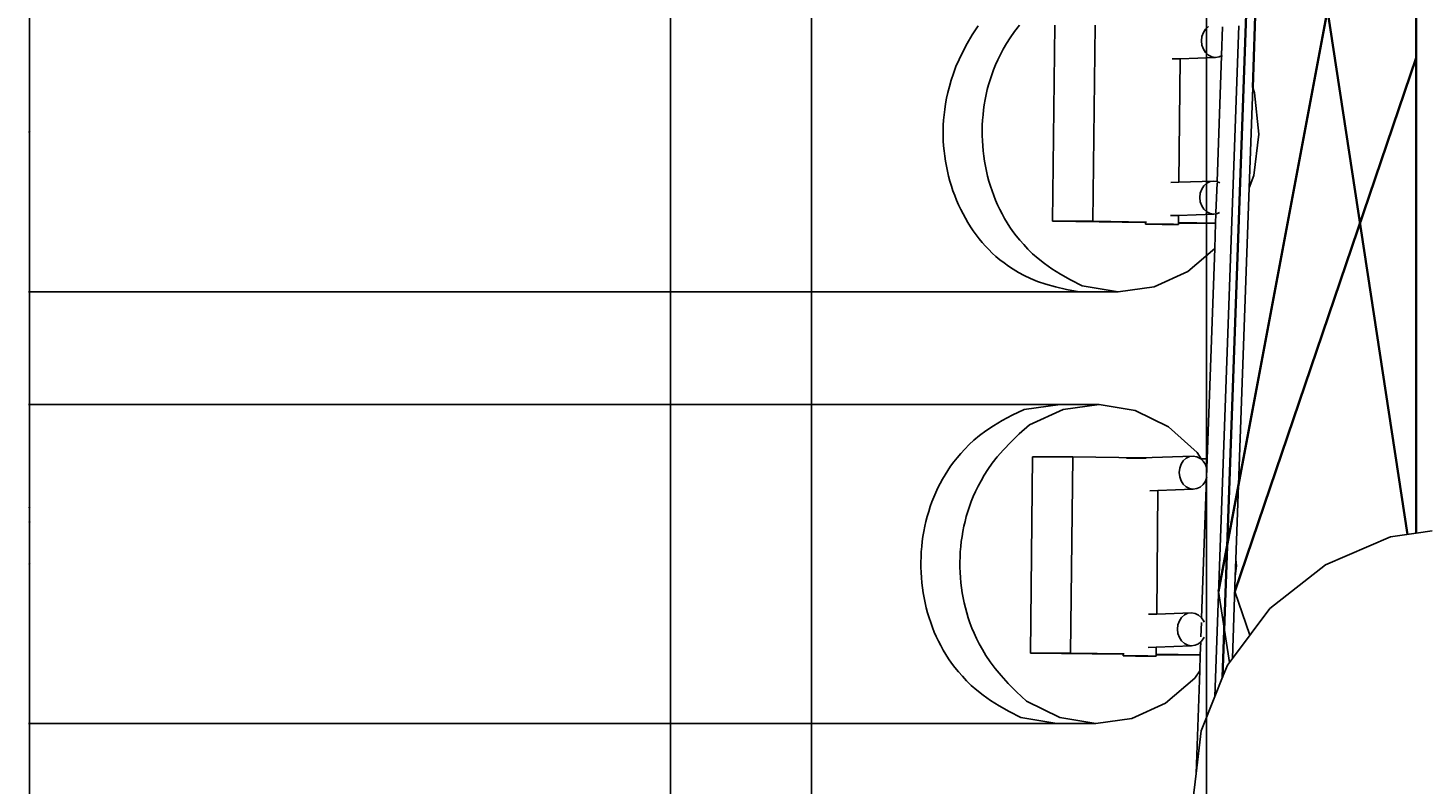
# Model space of a CAD drawing. Units: inches. Extents: x 3780 to 4301, y 1637 to 4224.
# Tile 5 of 8: x 3781 to 4040, y 3542 to 3682. Entities that reach past the tile are written whole.
import ezdxf

# ---------------------------------------------------------------- set-up
doc = ezdxf.new("R2010")
doc.units = ezdxf.units.IN
for name, color, linetype, lineweight in [('A-ANNO-DIMS', 2, 'Continuous', 18), ('E-COMM-DISH', 3, 'Continuous', 25), ('S-TOWR', 7, 'Continuous', 35)]:
    doc.layers.add(name, color=color, linetype=linetype, lineweight=lineweight)
doc.styles.get("Standard").update_dxf_attribs({"font": 'arial.ttf'})
doc.dimstyles.get("Standard").update_dxf_attribs({"dimtxt": 0.18, "dimasz": 0.18, "dimexe": 0.18, "dimexo": 0.0625, "dimgap": 0.09, "dimtad": 0, "dimtih": 1, "dimtoh": 1, "dimdec": 4, "dimzin": 0, "dimdsep": 46, "dimtxsty": 'Standard', "dimcen": 0.09, "dimadec": 0, "dimazin": 0, "dimtfac": 1, "dimtdec": 4, "dimtofl": 0, "dimtmove": 0, "dimatfit": 3, "dimfxl": 1, "dimtolj": 1, "dimtzin": 0, "dimarcsym": 0})

# ---------------------------------------------------------------- blocks, each defined once
blk = doc.blocks.new('*D11')
at = {"layer": 'A-ANNO-DIMS', "color": 0, "lineweight": -2, "transparency": 16777216}
for p, q in [((3916.19, 4105.28), (3780.66, 4105.28)), ((3780.84, 4105.1), (3780.84, 2930.44)), ((3780.84, 1755.43), (3780.84, 2930.08)), ((3934.09, 1755.25), (3780.66, 1755.25))]:
    blk.add_line(p, q, dxfattribs=at)
at = {"layer": 'A-ANNO-DIMS', "color": 0, "transparency": 16777216}
for points in [[(3780.81, 4105.1), (3780.87, 4105.1), (3780.84, 4105.28)], [(3780.81, 1755.43), (3780.87, 1755.43), (3780.84, 1755.25)]]:
    blk.add_solid(points, dxfattribs=at)
at = {"layer": 'Defpoints', "color": 0, "transparency": 16777216}
for p in [(3780.84, 4105.28), (3916.25, 4105.28), (3934.15, 1755.25)]:
    blk.add_point(p, dxfattribs=at)
at = {"layer": 'A-ANNO-DIMS', "color": 0, "transparency": 16777216, "insert": (3780.84, 2930.26), "char_height": 0.18, "attachment_point": 5}
blk.add_mtext('\\A1;2350', dxfattribs=at)
blk = doc.blocks.new('*D21')
at = {"layer": 'A-ANNO-DIMS', "color": 0, "lineweight": -2, "transparency": 16777216}
for p, q in [((4010.55, 3901.46), (4300.89, 3901.46)), ((4300.71, 3901.28), (4300.71, 3685.65)), ((4300.71, 3469.64), (4300.71, 3685.28)), ((4044.72, 3469.46), (4300.89, 3469.46))]:
    blk.add_line(p, q, dxfattribs=at)
at = {"layer": 'A-ANNO-DIMS', "color": 0, "transparency": 16777216}
for points in [[(4300.68, 3901.28), (4300.74, 3901.28), (4300.71, 3901.46)], [(4300.68, 3469.64), (4300.74, 3469.64), (4300.71, 3469.46)]]:
    blk.add_solid(points, dxfattribs=at)
at = {"layer": 'Defpoints', "color": 0, "transparency": 16777216}
for p in [(4010.49, 3901.46), (4300.71, 3901.46), (4044.66, 3469.46)]:
    blk.add_point(p, dxfattribs=at)
at = {"layer": 'A-ANNO-DIMS', "color": 0, "transparency": 16777216, "insert": (4300.71, 3685.46), "char_height": 0.18, "attachment_point": 5}
blk.add_mtext('\\A1;432', dxfattribs=at)
blk = doc.blocks.new('*D22')
at = {"layer": 'A-ANNO-DIMS', "color": 0, "lineweight": -2, "transparency": 16777216}
for p, q in [((3900.05, 3694.01), (3900.05, 1636.57)), ((4181.5, 3694.01), (4181.5, 1636.57)), ((3900.23, 1636.75), (4040.31, 1636.75)), ((4181.32, 1636.75), (4041.24, 1636.75))]:
    blk.add_line(p, q, dxfattribs=at)
at = {"layer": 'A-ANNO-DIMS', "color": 0, "transparency": 16777216}
for points in [[(3900.23, 1636.78), (3900.23, 1636.72), (3900.05, 1636.75)], [(4181.32, 1636.78), (4181.32, 1636.72), (4181.5, 1636.75)]]:
    blk.add_solid(points, dxfattribs=at)
at = {"layer": 'Defpoints', "color": 0, "transparency": 16777216}
for p in [(3900.05, 3694.07), (4181.5, 3694.07), (4181.5, 1636.75)]:
    blk.add_point(p, dxfattribs=at)
at = {"layer": 'A-ANNO-DIMS', "color": 0, "transparency": 16777216, "insert": (4040.77, 1636.75), "char_height": 0.18, "attachment_point": 5}
blk.add_mtext('\\A1;281.45', dxfattribs=at)
blk = doc.blocks.new('*D28')
at = {"layer": 'A-ANNO-DIMS', "color": 0, "lineweight": -2, "transparency": 16777216}
for p, q in [((3926.17, 3691.91), (3780.66, 3691.91)), ((3780.84, 3691.73), (3780.84, 3590.48)), ((3780.84, 3488.87), (3780.84, 3590.12)), ((4048.31, 3488.69), (3780.66, 3488.69))]:
    blk.add_line(p, q, dxfattribs=at)
at = {"layer": 'A-ANNO-DIMS', "color": 0, "transparency": 16777216}
for points in [[(3780.81, 3691.73), (3780.87, 3691.73), (3780.84, 3691.91)], [(3780.81, 3488.87), (3780.87, 3488.87), (3780.84, 3488.69)]]:
    blk.add_solid(points, dxfattribs=at)
at = {"layer": 'Defpoints', "color": 0, "transparency": 16777216}
for p in [(3780.84, 3691.91), (3926.23, 3691.91), (4048.37, 3488.69)]:
    blk.add_point(p, dxfattribs=at)
at = {"layer": 'A-ANNO-DIMS', "color": 0, "transparency": 16777216, "insert": (3780.84, 3590.3), "char_height": 0.18, "attachment_point": 5}
blk.add_mtext('\\A1;203.2', dxfattribs=at)
blk = doc.blocks.new('*D43')
at = {"layer": 'A-ANNO-DIMS', "color": 0, "lineweight": -2, "transparency": 16777216}
for p, q in [((3983.82, 3692.42), (3780.66, 3692.42)), ((3780.84, 3692.24), (3780.84, 3662.96)), ((3780.84, 3633.31), (3780.84, 3662.6)), ((3983.19, 3633.13), (3780.66, 3633.13))]:
    blk.add_line(p, q, dxfattribs=at)
at = {"layer": 'A-ANNO-DIMS', "color": 0, "transparency": 16777216}
for points in [[(3780.81, 3692.24), (3780.87, 3692.24), (3780.84, 3692.42)], [(3780.81, 3633.31), (3780.87, 3633.31), (3780.84, 3633.13)]]:
    blk.add_solid(points, dxfattribs=at)
at = {"layer": 'Defpoints', "color": 0, "transparency": 16777216}
for p in [(3983.89, 3692.42), (3780.84, 3633.13), (3983.25, 3633.13)]:
    blk.add_point(p, dxfattribs=at)
at = {"layer": 'A-ANNO-DIMS', "color": 0, "transparency": 16777216, "insert": (3780.84, 3662.78), "char_height": 0.18, "attachment_point": 5}
blk.add_mtext('\\A1;59.29', dxfattribs=at)
blk = doc.blocks.new('*D44')
at = {"layer": 'A-ANNO-DIMS', "color": 0, "lineweight": -2, "transparency": 16777216}
for p, q in [((3972.42, 3612.19), (3780.66, 3612.19)), ((3780.84, 3612.01), (3780.84, 3582.73)), ((3780.84, 3553.08), (3780.84, 3582.36)), ((3971.79, 3552.9), (3780.66, 3552.9))]:
    blk.add_line(p, q, dxfattribs=at)
at = {"layer": 'A-ANNO-DIMS', "color": 0, "transparency": 16777216}
for points in [[(3780.81, 3612.01), (3780.87, 3612.01), (3780.84, 3612.19)], [(3780.81, 3553.08), (3780.87, 3553.08), (3780.84, 3552.9)]]:
    blk.add_solid(points, dxfattribs=at)
at = {"layer": 'Defpoints', "color": 0, "transparency": 16777216}
for p in [(3972.48, 3612.19), (3780.84, 3552.9), (3971.85, 3552.9)]:
    blk.add_point(p, dxfattribs=at)
at = {"layer": 'A-ANNO-DIMS', "color": 0, "transparency": 16777216, "insert": (3780.84, 3582.55), "char_height": 0.18, "attachment_point": 5}
blk.add_mtext('\\A1;59.29', dxfattribs=at)
blk = doc.blocks.new('*D45')
at = {"layer": 'A-ANNO-DIMS', "color": 0, "lineweight": -2, "transparency": 16777216}
for p, q in [((3971.79, 3552.9), (3780.66, 3552.9)), ((3780.84, 3552.72), (3780.84, 3520.98)), ((3780.84, 3488.87), (3780.84, 3520.61)), ((4048.31, 3488.69), (3780.66, 3488.69))]:
    blk.add_line(p, q, dxfattribs=at)
at = {"layer": 'A-ANNO-DIMS', "color": 0, "transparency": 16777216}
for points in [[(3780.81, 3552.72), (3780.87, 3552.72), (3780.84, 3552.9)], [(3780.81, 3488.87), (3780.87, 3488.87), (3780.84, 3488.69)]]:
    blk.add_solid(points, dxfattribs=at)
at = {"layer": 'Defpoints', "color": 0, "transparency": 16777216}
for p in [(3780.84, 3552.9), (3971.85, 3552.9), (4048.37, 3488.69)]:
    blk.add_point(p, dxfattribs=at)
at = {"layer": 'A-ANNO-DIMS', "color": 0, "transparency": 16777216, "insert": (3780.84, 3520.8), "char_height": 0.18, "attachment_point": 5}
blk.add_mtext('\\A1;64.21', dxfattribs=at)
blk = doc.blocks.new('*D46')
at = {"layer": 'A-ANNO-DIMS', "color": 0, "lineweight": -2, "transparency": 16777216}
for p, q in [((3983.19, 3633.13), (3780.66, 3633.13)), ((3780.84, 3632.95), (3780.84, 3593.2)), ((3780.84, 3553.08), (3780.84, 3592.84)), ((3971.79, 3552.9), (3780.66, 3552.9))]:
    blk.add_line(p, q, dxfattribs=at)
at = {"layer": 'A-ANNO-DIMS', "color": 0, "transparency": 16777216}
for points in [[(3780.81, 3632.95), (3780.87, 3632.95), (3780.84, 3633.13)], [(3780.81, 3553.08), (3780.87, 3553.08), (3780.84, 3552.9)]]:
    blk.add_solid(points, dxfattribs=at)
at = {"layer": 'Defpoints', "color": 0, "transparency": 16777216}
for p in [(3780.84, 3633.13), (3983.25, 3633.13), (3971.85, 3552.9)]:
    blk.add_point(p, dxfattribs=at)
at = {"layer": 'A-ANNO-DIMS', "color": 0, "transparency": 16777216, "insert": (3780.84, 3593.02), "char_height": 0.18, "attachment_point": 5}
blk.add_mtext('\\A1;80.23', dxfattribs=at)
blk = doc.blocks.new('*D48')
at = {"layer": 'A-ANNO-DIMS', "color": 0, "lineweight": -2, "transparency": 16777216}
for p, q in [((3926.23, 3245.63), (3926.23, 4223.96)), ((3926.41, 4223.78), (3962.66, 4223.78)), ((3999.55, 4223.78), (3963.31, 4223.78)), ((3999.73, 3245.63), (3999.73, 4223.96))]:
    blk.add_line(p, q, dxfattribs=at)
at = {"layer": 'A-ANNO-DIMS', "color": 0, "transparency": 16777216}
for points in [[(3926.41, 4223.81), (3926.41, 4223.75), (3926.23, 4223.78)], [(3999.55, 4223.81), (3999.55, 4223.75), (3999.73, 4223.78)]]:
    blk.add_solid(points, dxfattribs=at)
at = {"layer": 'Defpoints', "color": 0, "transparency": 16777216}
for p in [(3999.73, 4223.78), (3926.23, 3245.56), (3999.73, 3245.56)]:
    blk.add_point(p, dxfattribs=at)
at = {"layer": 'A-ANNO-DIMS', "color": 0, "transparency": 16777216, "insert": (3962.98, 4223.78), "char_height": 0.18, "attachment_point": 5}
blk.add_mtext('\\A1;73.5', dxfattribs=at)
blk = doc.blocks.new('*D49')
at = {"layer": 'A-ANNO-DIMS', "color": 0, "lineweight": -2, "transparency": 16777216}
for p, q in [((3999.73, 3245.63), (3999.73, 4223.96)), ((3999.91, 4223.78), (4036.16, 4223.78)), ((4073.05, 4223.78), (4036.81, 4223.78)), ((4073.23, 3245.63), (4073.23, 4223.96))]:
    blk.add_line(p, q, dxfattribs=at)
at = {"layer": 'A-ANNO-DIMS', "color": 0, "transparency": 16777216}
for points in [[(3999.91, 4223.81), (3999.91, 4223.75), (3999.73, 4223.78)], [(4073.05, 4223.81), (4073.05, 4223.75), (4073.23, 4223.78)]]:
    blk.add_solid(points, dxfattribs=at)
at = {"layer": 'Defpoints', "color": 0, "transparency": 16777216}
for p in [(4073.23, 4223.78), (3999.73, 3245.56), (4073.23, 3245.56)]:
    blk.add_point(p, dxfattribs=at)
at = {"layer": 'A-ANNO-DIMS', "color": 0, "transparency": 16777216, "insert": (4036.48, 4223.78), "char_height": 0.18, "attachment_point": 5}
blk.add_mtext('\\A1;73.5', dxfattribs=at)

msp = doc.modelspace()

# ---------------------------------------------------------------- linework, layer by layer
at = {"layer": 'E-COMM-DISH'}
for p, q in [((3971.4759, 3682.6716), (3971.0873, 3646.2373)), ((3978.9667, 3682.6716), (3978.5781, 3646.2373)), ((3999.5309, 3681.9506), (3999.1145, 3681.3201)), ((4000.0735, 3682.4316), (3999.5309, 3681.9506)), ((4001.2675, 3557.9436), (4005.6996, 3682.5582)), ((4002.5039, 3677.0562), (4002.6939, 3682.398)), ((3998.8529, 3680.583), (3998.7638, 3679.7895)), ((3998.7638, 3679.7895), (3998.8532, 3678.9938)), ((3999.1145, 3681.3201), (3998.8529, 3680.583)), ((3998.8532, 3678.9938), (3999.1151, 3678.2499)), ((3994.8223, 3676.4558), (3993.3061, 3676.4026)), ((3994.5773, 3653.4864), (3994.8223, 3676.4558)), ((4001.3848, 3676.6858), (3994.8223, 3676.4558)), ((3999.1151, 3678.2499), (3999.5317, 3677.6087)), ((3999.5317, 3677.6087), (4000.0745, 3677.1139)), ((4000.0745, 3677.1139), (4000.7065, 3676.7991)), ((4000.7065, 3676.7991), (4001.3848, 3676.6858)), ((4001.3848, 3676.6858), (4002.063, 3676.7817)), ((4001.6702, 3653.6144), (4002.5015, 3676.9889)), ((4002.063, 3676.7817), (4002.5015, 3676.9889)), ((4002.5015, 3676.9889), (4002.6491, 3677.0586)), ((4007.6297, 3652.4757), (4008.2926, 3671.1131)), ((4008.2926, 3671.1131), (4008.6463, 3670.1)), ((4008.6463, 3670.1), (4009.4462, 3662.4153)), ((4009.4462, 3662.4153), (4008.4826, 3654.7554)), ((3994.5773, 3653.4864), (3993.0549, 3653.4331)), ((4001.0731, 3653.7141), (3994.5773, 3653.4864)), ((3999.763, 3653.3196), (3999.2204, 3652.8386)), ((4000.3949, 3653.6182), (3999.763, 3653.3196)), ((4001.0731, 3653.7141), (4000.3949, 3653.6182)), ((4001.6702, 3653.6144), (4001.0731, 3653.7141)), ((4001.4647, 3647.8375), (4001.6611, 3653.3589)), ((4001.7514, 3653.6008), (4001.6702, 3653.6144)), ((4002.1776, 3653.3885), (4001.7514, 3653.6008)), ((4008.4826, 3654.7554), (4007.6297, 3652.4757)), ((3998.5424, 3651.471), (3998.4533, 3650.6775)), ((3998.4533, 3650.6775), (3998.5427, 3649.8818)), ((3998.804, 3652.2081), (3998.5424, 3651.471)), ((3999.2204, 3652.8386), (3998.804, 3652.2081)), ((4005.1742, 3583.436), (4007.6297, 3652.4757)), ((3998.5427, 3649.8818), (3998.8046, 3649.1379)), ((3998.8046, 3649.1379), (3999.2212, 3648.4967)), ((3999.2212, 3648.4967), (3999.764, 3648.0019)), ((3999.764, 3648.0019), (4000.3961, 3647.6871)), ((4001.7525, 3647.6697), (4002.1312, 3647.8486)), ((3971.0873, 3646.2373), (3988.356, 3645.9956)), ((3971.0873, 3646.2373), (3978.5781, 3646.2373)), ((3978.5781, 3646.2373), (3988.5571, 3646.0977)), ((3988.3531, 3645.7237), (3988.356, 3645.9956)), ((3988.4466, 3645.7274), (3988.3531, 3645.7237)), ((3988.3531, 3645.7237), (3988.4688, 3645.7177)), ((3988.356, 3645.9956), (3988.357, 3646.0934)), ((3988.743, 3645.7287), (3988.4466, 3645.7274)), ((3988.4688, 3645.7177), (3988.7858, 3645.71)), ((3989.2221, 3645.7274), (3988.743, 3645.7287)), ((3988.7858, 3645.71), (3989.2826, 3645.7009)), ((3989.8512, 3645.7237), (3989.2221, 3645.7274)), ((3989.2826, 3645.7009), (3989.9253, 3645.6912)), ((3990.5875, 3645.7177), (3989.8512, 3645.7237)), ((3989.9253, 3645.6912), (3990.6701, 3645.6815)), ((3991.3807, 3645.71), (3990.5875, 3645.7177)), ((3990.6701, 3645.6815), (3991.4662, 3645.6724)), ((3992.1768, 3645.7009), (3991.3807, 3645.71)), ((3991.4662, 3645.6724), (3992.2595, 3645.6647)), ((3992.9216, 3645.6912), (3992.1768, 3645.7009)), ((3992.2595, 3645.6647), (3992.9957, 3645.6587)), ((3993.5643, 3645.6815), (3992.9216, 3645.6912)), ((3994.5118, 3647.3438), (3992.9956, 3647.2906)), ((3992.9957, 3645.6587), (3993.6248, 3645.655)), ((3994.0611, 3645.6724), (3993.5643, 3645.6815)), ((3993.6248, 3645.655), (3994.1039, 3645.6537)), ((3994.3782, 3645.6647), (3994.0611, 3645.6724)), ((3994.1039, 3645.6537), (3994.4003, 3645.655)), ((3994.4939, 3645.6587), (3994.3782, 3645.6647)), ((3994.4003, 3645.655), (3994.4939, 3645.6587)), ((3994.4939, 3645.6587), (3994.4965, 3645.9097)), ((3994.4965, 3645.9097), (3994.4977, 3646.0145)), ((3994.4965, 3645.9097), (3996.8607, 3645.8766)), ((3994.4977, 3646.0145), (3994.5118, 3647.3438)), ((3994.4977, 3646.0145), (4001.3965, 3645.9179)), ((4001.0743, 3647.5738), (3994.5118, 3647.3438)), ((3996.8607, 3645.8766), (4001.395, 3645.8766)), ((4000.3961, 3647.6871), (4001.0743, 3647.5738)), ((4001.0743, 3647.5738), (4001.4573, 3647.6279)), ((4001.2288, 3641.2049), (4001.395, 3645.8766)), ((4001.395, 3645.8766), (4001.3965, 3645.9179)), ((4001.3965, 3645.9179), (4001.4573, 3647.6279)), ((4001.4573, 3647.6279), (4001.7525, 3647.6697)), ((4001.2288, 3641.2049), (3996.2341, 3636.9244)), ((3999.8377, 3602.0904), (4001.2288, 3641.2049)), ((3996.2341, 3636.9244), (3989.9617, 3634.0504)), ((3983.2536, 3633.1341), (3975.9933, 3633.1341)), ((3983.2536, 3633.1341), (3976.567, 3634.2379)), ((3989.9617, 3634.0504), (3983.2536, 3633.1341)), ((3965.7759, 3611.2736), (3972.4839, 3612.1899)), ((3979.7442, 3612.1899), (3972.4839, 3612.1899)), ((3973.0361, 3611.2736), (3979.7442, 3612.1899)), ((3979.7442, 3612.1899), (3986.4308, 3611.0861)), ((3966.7637, 3608.3995), (3973.0361, 3611.2736)), ((3986.4308, 3611.0861), (3992.6401, 3608.0373)), ((3992.6401, 3608.0373), (3997.949, 3603.2514)), ((3967.3342, 3602.4405), (3966.9457, 3566.0062)), ((3967.3342, 3602.4405), (3974.825, 3602.4405)), ((3974.825, 3602.4405), (3974.4364, 3566.0062)), ((3987.6941, 3602.2604), (3974.825, 3602.4405)), ((3984.9933, 3602.2458), (3984.8034, 3602.245)), ((3985.4724, 3602.2445), (3984.9933, 3602.2458)), ((3986.1015, 3602.2408), (3985.4724, 3602.2445)), ((3986.8377, 3602.2348), (3986.1015, 3602.2408)), ((3987.2907, 3602.2304), (3986.8377, 3602.2348)), ((3987.44, 3602.2515), (3987.2907, 3602.2304)), ((3987.631, 3602.2271), (3987.2907, 3602.2304)), ((3987.6941, 3602.2604), (3987.44, 3602.2515)), ((3988.4271, 3602.218), (3987.631, 3602.2271)), ((3997.2419, 3602.595), (3987.6941, 3602.2604)), ((3988.4822, 3602.2159), (3988.4271, 3602.218)), ((3988.4822, 3602.2159), (3988.4919, 3602.2172)), ((3995.3892, 3601.7195), (3994.9729, 3601.089)), ((3995.9318, 3602.2005), (3995.3892, 3601.7195)), ((3996.5637, 3602.4991), (3995.9318, 3602.2005)), ((3997.2419, 3602.595), (3996.5637, 3602.4991)), ((3997.9202, 3602.4817), (3997.2419, 3602.595)), ((3998.5522, 3602.1669), (3997.9202, 3602.4817)), ((3997.949, 3603.2514), (3998.6968, 3602.1064)), ((3998.6174, 3602.1075), (3998.5522, 3602.1669)), ((3999.0951, 3601.672), (3998.6174, 3602.1075)), ((3998.6968, 3602.1064), (3998.6174, 3602.1075)), ((3999.8377, 3602.0904), (3998.6968, 3602.1064)), ((3999.5116, 3601.0308), (3999.0951, 3601.672)), ((3999.7735, 3600.287), (3999.8377, 3602.0904)), ((3994.7112, 3600.3519), (3994.6221, 3599.5585)), ((3994.6221, 3599.5585), (3994.7115, 3598.7627)), ((3994.9729, 3601.089), (3994.7112, 3600.3519)), ((3994.7115, 3598.7627), (3994.9735, 3598.0189)), ((3998.7872, 3572.5559), (3999.7107, 3598.5199)), ((3999.7735, 3600.287), (3999.5116, 3601.0308)), ((3999.5122, 3597.9607), (3999.7107, 3598.5199)), ((3999.7107, 3598.5199), (3999.7599, 3598.6585)), ((3999.7157, 3598.6622), (3999.7735, 3600.287)), ((3990.6807, 3596.2247), (3989.1645, 3596.1716)), ((3990.4357, 3573.2554), (3990.6807, 3596.2247)), ((3997.2431, 3596.4547), (3990.6807, 3596.2247)), ((3994.9735, 3598.0189), (3995.39, 3597.3777)), ((3995.39, 3597.3777), (3995.9328, 3596.8828)), ((3995.9328, 3596.8828), (3996.5649, 3596.568)), ((3996.5649, 3596.568), (3997.2431, 3596.4547)), ((3997.2431, 3596.4547), (3997.9213, 3596.5506)), ((3997.9213, 3596.5506), (3998.5533, 3596.8492)), ((3998.5533, 3596.8492), (3999.0959, 3597.3302)), ((3999.0959, 3597.3302), (3999.5122, 3597.9607)), ((4038.6622, 3588.2865), (4033.8999, 3587.6003)), ((4041.6622, 3588.7189), (4038.6622, 3588.2865)), ((4033.8999, 3587.6003), (4021.8079, 3582.4174)), ((4005.0608, 3580.2468), (4005.1742, 3583.436)), ((4005.1742, 3583.436), (4005.3045, 3582.1843)), ((4005.3045, 3582.1843), (4005.0608, 3580.2468)), ((4021.8079, 3582.4174), (4011.4692, 3574.2814)), ((4004.5181, 3564.9893), (4005.0608, 3580.2468)), ((4001.9618, 3577.4644), (4003.9709, 3564.2578)), ((4004.9618, 3577.4644), (4007.7383, 3569.294)), ((3990.4357, 3573.2554), (3988.9132, 3573.202)), ((3996.9315, 3573.483), (3990.4357, 3573.2554)), ((3995.0787, 3572.6075), (3994.6624, 3571.977)), ((3995.6213, 3573.0885), (3995.0787, 3572.6075)), ((3996.2533, 3573.3871), (3995.6213, 3573.0885)), ((3996.9315, 3573.483), (3996.2533, 3573.3871)), ((3997.6097, 3573.3697), (3996.9315, 3573.483)), ((3998.2418, 3573.0549), (3997.6097, 3573.3697)), ((3998.7846, 3572.56), (3998.2418, 3573.0549)), ((3998.7872, 3572.5559), (3998.7846, 3572.56)), ((3999.2011, 3571.9188), (3998.7872, 3572.5559)), ((4011.4692, 3574.2814), (4004.5181, 3564.9893)), ((3994.4007, 3571.2399), (3994.3116, 3570.4465)), ((3994.3116, 3570.4465), (3994.401, 3569.6507)), ((3994.6624, 3571.977), (3994.4007, 3571.2399)), ((3998.6607, 3568.9989), (3998.7558, 3571.6711)), ((3999.2612, 3571.7483), (3999.2011, 3571.9188)), ((3996.9326, 3567.3427), (3990.3702, 3567.1127)), ((3994.401, 3569.6507), (3994.663, 3568.9069)), ((3994.663, 3568.9069), (3995.0795, 3568.2657)), ((3995.0795, 3568.2657), (3995.6223, 3567.7708)), ((3995.6223, 3567.7708), (3996.2544, 3567.456)), ((3996.2544, 3567.456), (3996.9326, 3567.3427)), ((3996.9326, 3567.3427), (3997.6108, 3567.4386)), ((3997.6108, 3567.4386), (3998.2428, 3567.7372)), ((3998.2428, 3567.7372), (3998.628, 3568.0787)), ((3998.5423, 3565.6688), (3998.628, 3568.0787)), ((3998.628, 3568.0787), (3998.7854, 3568.2182)), ((3998.7854, 3568.2182), (3999.2017, 3568.8487)), ((3999.2017, 3568.8487), (3999.2377, 3568.9501)), ((3966.9457, 3566.0062), (3984.2143, 3565.7645)), ((3966.9457, 3566.0062), (3974.4364, 3566.0062)), ((3974.4364, 3566.0062), (3984.4155, 3565.8666)), ((3984.2114, 3565.4926), (3984.2143, 3565.7645)), ((3984.305, 3565.4964), (3984.2114, 3565.4926)), ((3984.2114, 3565.4926), (3984.3271, 3565.4867)), ((3984.2143, 3565.7645), (3984.2154, 3565.8624)), ((3984.6014, 3565.4976), (3984.305, 3565.4964)), ((3984.3271, 3565.4867), (3984.6442, 3565.4789)), ((3985.0805, 3565.4964), (3984.6014, 3565.4976)), ((3984.6442, 3565.4789), (3985.141, 3565.4698)), ((3985.7096, 3565.4926), (3985.0805, 3565.4964)), ((3985.141, 3565.4698), (3985.7837, 3565.4601)), ((3986.4458, 3565.4867), (3985.7096, 3565.4926)), ((3985.7837, 3565.4601), (3986.5284, 3565.4504)), ((3987.239, 3565.4789), (3986.4458, 3565.4867)), ((3986.5284, 3565.4504), (3987.3246, 3565.4414)), ((3988.0352, 3565.4698), (3987.239, 3565.4789)), ((3987.3246, 3565.4414), (3988.1178, 3565.4336)), ((3988.78, 3565.4601), (3988.0352, 3565.4698)), ((3988.1178, 3565.4336), (3988.854, 3565.4276)), ((3989.4227, 3565.4504), (3988.78, 3565.4601)), ((3990.3702, 3567.1127), (3988.854, 3567.0596)), ((3988.854, 3565.4276), (3989.4831, 3565.4239)), ((3989.9195, 3565.4414), (3989.4227, 3565.4504)), ((3989.4831, 3565.4239), (3989.9622, 3565.4226)), ((3990.2365, 3565.4336), (3989.9195, 3565.4414)), ((3989.9622, 3565.4226), (3990.2586, 3565.4239)), ((3990.3522, 3565.4276), (3990.2365, 3565.4336)), ((3990.2586, 3565.4239), (3990.3522, 3565.4276)), ((3990.3522, 3565.4276), (3990.3549, 3565.6786)), ((3990.3549, 3565.6786), (3990.356, 3565.7834)), ((3990.3549, 3565.6786), (3992.719, 3565.6455)), ((3990.356, 3565.7834), (3990.3702, 3567.1127)), ((3990.356, 3565.7834), (3998.5423, 3565.6688)), ((3992.719, 3565.6455), (3998.5415, 3565.6455)), ((3998.4363, 3562.6896), (3998.5415, 3565.6455)), ((3998.5415, 3565.6455), (3998.5423, 3565.6688)), ((4004.5181, 3564.9893), (4003.5885, 3563.7466)), ((3998.4363, 3562.6896), (3997.5019, 3561.3293)), ((3997.7575, 3543.6033), (3998.4363, 3562.6896)), ((4003.5885, 3563.7466), (4002.6934, 3561.5086)), ((3997.5019, 3561.3293), (3992.0925, 3556.6934)), ((4002.6934, 3561.5086), (4001.2675, 3557.9436)), ((3972.4254, 3554.0068), (3966.2161, 3557.0556)), ((4001.2675, 3557.9436), (3998.7028, 3551.531)), ((3992.0925, 3556.6934), (3985.82, 3553.8193)), ((3971.8516, 3552.903), (3965.1651, 3554.0068)), ((3979.1119, 3552.903), (3971.8516, 3552.903)), ((3979.1119, 3552.903), (3972.4254, 3554.0068)), ((3985.82, 3553.8193), (3979.1119, 3552.903)), ((3998.7028, 3551.531), (3997.7575, 3543.6033)), ((3997.7575, 3543.6033), (3997.1451, 3538.4672))]:
    msp.add_line(p, q, dxfattribs=at)
for points in [[(3975.9933, 3633.1341), (3973.6481, 3633.567), (3971.6045, 3634.0348), (3969.8284, 3634.533), (3968.2856, 3635.0571), (3966.942, 3635.6025), (3965.7635, 3636.1649), (3964.7159, 3636.7396), (3963.765, 3637.3221), (3962.8814, 3637.9091), (3962.0551, 3638.5017), (3961.2807, 3639.1024), (3960.5527, 3639.7134), (3959.8659, 3640.3371), (3959.2149, 3640.9758), (3958.5944, 3641.6319), (3957.9989, 3642.3077), (3957.4241, 3643.005), (3956.8696, 3643.7236), (3956.3358, 3644.4625), (3955.8235, 3645.221), (3955.3329, 3645.9982), (3954.8649, 3646.7934), (3954.4197, 3647.6057), (3953.9981, 3648.4342), (3953.6004, 3649.2782), (3953.2271, 3650.1367), (3952.8785, 3651.0087), (3952.555, 3651.8933), (3952.2568, 3652.7895), (3951.9843, 3653.6963), (3951.7378, 3654.6129), (3951.5177, 3655.5382), (3951.3243, 3656.4714), (3951.1577, 3657.4113), (3951.018, 3658.3569), (3950.9053, 3659.3073), (3950.8198, 3660.2614), (3950.7614, 3661.2181), (3950.7305, 3662.1765), (3950.7269, 3663.1356), (3950.7514, 3664.0954), (3950.8058, 3665.0608), (3950.8927, 3666.0376), (3951.0146, 3667.0319), (3951.174, 3668.0494), (3951.3732, 3669.0962), (3951.6148, 3670.1782), (3951.9013, 3671.3013), (3952.2373, 3672.4716), (3952.6366, 3673.6958), (3953.1149, 3674.9807), (3953.6882, 3676.3334), (3954.3723, 3677.7606), (3955.1832, 3679.2692), (3956.1368, 3680.8661), (3957.2488, 3682.5582)], [(3976.567, 3634.2379), (3974.3995, 3635.3514), (3972.5312, 3636.4092), (3970.9282, 3637.417), (3969.5564, 3638.3807), (3968.3819, 3639.3059), (3967.3706, 3640.1985), (3966.4885, 3641.0643), (3965.7016, 3641.9089), (3964.9807, 3642.7378), (3964.3165, 3643.5553), (3963.7041, 3644.3651), (3963.139, 3645.1711), (3962.6166, 3645.9772), (3962.132, 3646.7872), (3961.6808, 3647.6049), (3961.2583, 3648.4342), (3960.8607, 3649.2782), (3960.4874, 3650.1367), (3960.1388, 3651.0087), (3959.8152, 3651.8933), (3959.5171, 3652.7895), (3959.2446, 3653.6963), (3958.9981, 3654.6129), (3958.778, 3655.5382), (3958.5846, 3656.4714), (3958.418, 3657.4113), (3958.2783, 3658.3569), (3958.1656, 3659.3073), (3958.08, 3660.2614), (3958.0217, 3661.2181), (3957.9907, 3662.1765), (3957.9872, 3663.1356), (3958.0112, 3664.0943), (3958.0626, 3665.0515), (3958.1413, 3666.0064), (3958.2472, 3666.9578), (3958.3801, 3667.9047), (3958.5399, 3668.8462), (3958.7265, 3669.7811), (3958.9398, 3670.7085), (3959.1802, 3671.6284), (3959.4509, 3672.5448), (3959.7556, 3673.4625), (3960.098, 3674.3868), (3960.4818, 3675.3224), (3960.9108, 3676.2745), (3961.3886, 3677.2479), (3961.919, 3678.2478), (3962.5105, 3679.2807), (3963.1902, 3680.3598), (3963.9899, 3681.4998), (3964.9416, 3682.7155)], [(3965.1651, 3554.0068), (3962.9976, 3555.1203), (3961.1293, 3556.1781), (3959.5263, 3557.1859), (3958.1545, 3558.1496), (3956.9799, 3559.0748), (3955.9686, 3559.9675), (3955.0865, 3560.8332), (3954.2996, 3561.6778), (3953.5788, 3562.5068), (3952.9145, 3563.3242), (3952.3022, 3564.134), (3951.7371, 3564.9401), (3951.2146, 3565.7461), (3950.7301, 3566.5561), (3950.2789, 3567.3738), (3949.8564, 3568.2032), (3949.4587, 3569.0471), (3949.0855, 3569.9056), (3948.7369, 3570.7776), (3948.4133, 3571.6622), (3948.1151, 3572.5584), (3947.8426, 3573.4653), (3947.5962, 3574.3818), (3947.3761, 3575.3072), (3947.1827, 3576.2403), (3947.016, 3577.1802), (3946.8763, 3578.1258), (3946.7637, 3579.0762), (3946.6781, 3580.0303), (3946.6198, 3580.987), (3946.5888, 3581.9455), (3946.5853, 3582.9045), (3946.6093, 3583.8632), (3946.6607, 3584.8205), (3946.7394, 3585.7753), (3946.8452, 3586.7267), (3946.9782, 3587.6736), (3947.138, 3588.6151), (3947.3246, 3589.55), (3947.5379, 3590.4775), (3947.7776, 3591.3964), (3948.0436, 3592.3058), (3948.3353, 3593.2047), (3948.6525, 3594.0923), (3948.9949, 3594.9676), (3949.3619, 3595.8296), (3949.7534, 3596.6773), (3950.169, 3597.5099), (3950.609, 3598.3272), (3951.0775, 3599.132), (3951.5792, 3599.9282), (3952.1187, 3600.7194), (3952.7008, 3601.5094), (3953.3302, 3602.3018), (3954.0117, 3603.1004), (3954.75, 3603.909), (3955.5547, 3604.7313), (3956.455, 3605.5721), (3957.4851, 3606.4361), (3958.679, 3607.3282), (3960.0709, 3608.2532), (3961.695, 3609.2159), (3963.5852, 3610.2211), (3965.7759, 3611.2736)], [(3966.2161, 3557.0556), (3964.374, 3558.7738), (3962.8083, 3560.3495), (3961.4876, 3561.7983), (3960.3803, 3563.1358), (3959.4548, 3564.3778), (3958.6796, 3565.5398), (3958.0232, 3566.6376), (3957.4539, 3567.6868), (3956.9449, 3568.7012), (3956.488, 3569.6877), (3956.0795, 3570.6515), (3955.7157, 3571.5976), (3955.3932, 3572.5312), (3955.1082, 3573.4572), (3954.8571, 3574.3808), (3954.6363, 3575.3072), (3954.4429, 3576.2403), (3954.2763, 3577.1802), (3954.1366, 3578.1258), (3954.0239, 3579.0762), (3953.9384, 3580.0303), (3953.8801, 3580.987), (3953.8491, 3581.9455), (3953.8455, 3582.9045), (3953.8695, 3583.8632), (3953.9209, 3584.8205), (3953.9996, 3585.7753), (3954.1055, 3586.7267), (3954.2384, 3587.6736), (3954.3983, 3588.6151), (3954.5849, 3589.55), (3954.7981, 3590.4775), (3955.0386, 3591.3974), (3955.3093, 3592.3137), (3955.6139, 3593.2315), (3955.9563, 3594.1557), (3956.3401, 3595.0913), (3956.7691, 3596.0434), (3957.2469, 3597.0169), (3957.7774, 3598.0167), (3958.3689, 3599.0497), (3959.0485, 3600.1287), (3959.8483, 3601.2687), (3960.8, 3602.4844), (3961.9355, 3603.7906), (3963.2867, 3605.202), (3964.8855, 3606.7334), (3966.7637, 3608.3995)]]:
    msp.add_lwpolyline(points, dxfattribs=at)
at = {"layer": 'S-TOWR'}
for p, q in [((4038.6622, 3588.2865), (4038.6622, 3751.5582)), ((4002.6934, 3561.5086), (4007.3312, 3691.9077)), ((4009.0321, 3691.9077), (4008.2926, 3671.1131)), ((4022.2326, 3685.4644), (4001.9618, 3577.4644)), ((4037.0512, 3588.0544), (4022.2326, 3685.4644)), ((4038.6622, 3676.6362), (4004.9618, 3577.4644))]:
    msp.add_line(p, q, dxfattribs=at)

# ---------------------------------------------------------------- dimensions: what is measured, and where the dimension line sits
at = {"layer": 'A-ANNO-DIMS'}
for base, p1, p2, override, picture, middle in [((3999.7315, 4223.7769), (3926.2315, 3245.5639), (3999.7315, 3245.5639), {"dimdec": 1, "dimlfac": 1, "dimrnd": 0, "dimzin": 0, "dimdsep": 46, "dimlunit": 2}, '*D48', (3962.9815, 4223.7769)), ((4073.2315, 4223.7769), (3999.7315, 3245.5639), (4073.2315, 3245.5639), {"dimdec": 1, "dimlfac": 1, "dimrnd": 0, "dimzin": 0, "dimdsep": 46, "dimlunit": 2}, '*D49', (4036.4815, 4223.7769)), ((4181.498, 1636.7487), (3900.0482, 3694.0677), (4181.498, 3694.0677), {"dimdec": 2, "dimlfac": 1, "dimrnd": 0, "dimzin": 0, "dimdsep": 46, "dimlunit": 2}, '*D22', (4040.7731, 1636.7487))]:
    dim = msp.add_linear_dim(base=base, p1=p1, p2=p2, dimstyle='Standard', override=override, dxfattribs=at)
    dim.commit()
    dim.dimension.update_dxf_attribs({"geometry": picture, "text_midpoint": middle})
for base, p1, p2, override, picture, middle in [((3780.8371, 4105.2769), (3934.1525, 1755.2487), (3916.252, 4105.2769), {"dimdec": 0, "dimlfac": 1, "dimrnd": 0, "dimzin": 0, "dimdsep": 46, "dimlunit": 2}, '*D11', (3780.8371, 2930.2628)), ((4300.7091, 3901.4644), (4044.6622, 3469.4644), (4010.4853, 3901.4644), {"dimdec": 0, "dimlfac": 1, "dimrnd": 0, "dimzin": 0, "dimdsep": 46, "dimlunit": 2}, '*D21', (4300.7091, 3685.4644)), ((3780.8371, 3633.1341), (3983.8859, 3692.421), (3983.2536, 3633.1341), {"dimdec": 2, "dimlfac": 1, "dimrnd": 0, "dimzin": 0, "dimdsep": 46, "dimlunit": 2}, '*D43', (3780.8371, 3662.7775)), ((3780.8371, 3691.9077), (4048.3735, 3488.689), (3926.2315, 3691.9077), {"dimdec": 1, "dimlfac": 1, "dimrnd": 0, "dimzin": 0, "dimdsep": 46, "dimlunit": 2}, '*D28', (3780.8371, 3590.2983)), ((3780.8371, 3633.1341), (3971.8516, 3552.903), (3983.2536, 3633.1341), {"dimdec": 2, "dimlfac": 1, "dimrnd": 0, "dimzin": 0, "dimdsep": 46, "dimlunit": 2}, '*D46', (3780.8371, 3593.0185)), ((3780.8371, 3552.903), (3972.4839, 3612.1899), (3971.8516, 3552.903), {"dimdec": 2, "dimlfac": 1, "dimrnd": 0, "dimzin": 0, "dimdsep": 46, "dimlunit": 2}, '*D44', (3780.8371, 3582.5464)), ((3780.8371, 3552.903), (4048.3735, 3488.689), (3971.8516, 3552.903), {"dimdec": 2, "dimlfac": 1, "dimrnd": 0, "dimzin": 0, "dimdsep": 46, "dimlunit": 2}, '*D45', (3780.8371, 3520.796))]:
    dim = msp.add_linear_dim(base=base, p1=p1, p2=p2, angle=90, dimstyle='Standard', override=override, dxfattribs=at)
    dim.commit()
    dim.dimension.update_dxf_attribs({"geometry": picture, "text_midpoint": middle})

doc.saveas('drawing.dxf')
